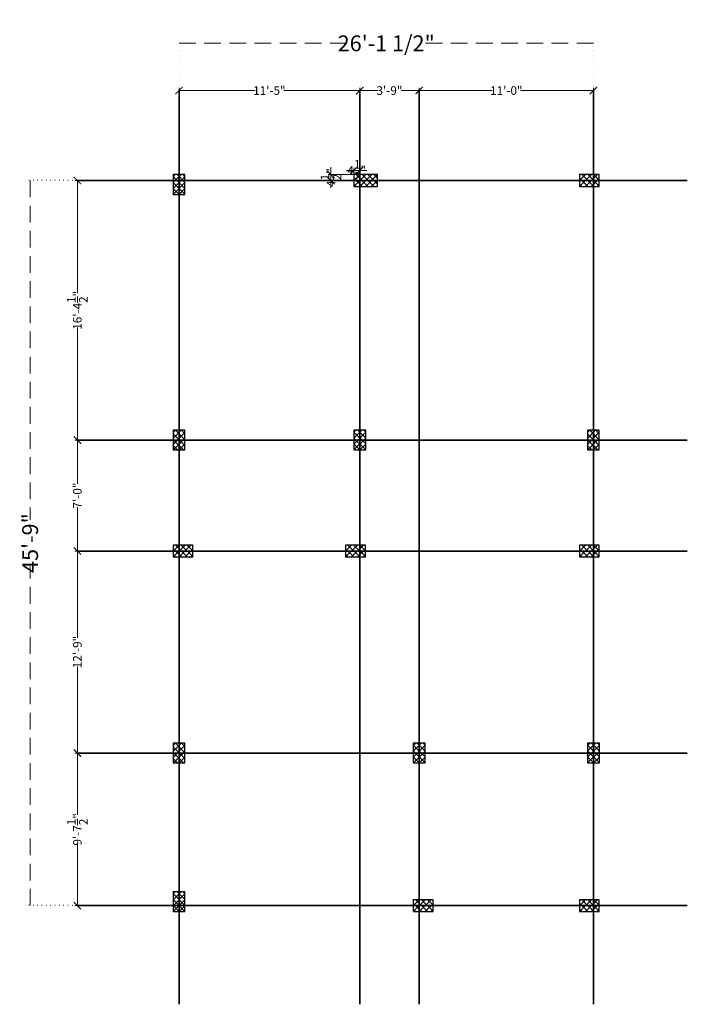
# Model space of a CAD drawing. Units: inches. Extents: x -16911 to -9621, y -48626 to -46270.
# Tile 9 of 20: x -13485 to -12980, y -47015 to -46270. Entities that reach past the tile are written whole.
import ezdxf

# ---------------------------------------------------------------- set-up
doc = ezdxf.new("R2010")
doc.units = ezdxf.units.IN
doc.linetypes.add('DASHED', pattern=[19.05, 12.7, -6.35])
doc.linetypes.add('DOT2', pattern=[3.175, 0, -3.175])
for name, color, linetype, lineweight in [('A-ANNO-DIMS', 2, 'Continuous', 13), ('A-WALL', 7, 'Continuous', 35), ('column', 12, 'Continuous', 30), ('S-COLS', 1, 'Continuous', 30)]:
    doc.layers.add(name, color=color, linetype=linetype, lineweight=lineweight)
doc.styles.add('style3', font='times.ttf')
doc.styles.add('style9', font='swisscl.ttf', dxfattribs={"height": 12})
doc.dimstyles.new('Dim9', dxfattribs={"dimtxt": 10, "dimasz": 0.199219, "dimexe": 1, "dimexo": 0.5, "dimgap": 1, "dimtad": 0, "dimdec": 1, "dimzin": 0, "dimdsep": 46, "dimlunit": 4, "dimtxsty": 'style9', "dimblk": 'ARCHTICK', "dimcen": 0.09, "dimclrd": 256, "dimclrt": 256, "dimadec": 0, "dimazin": 0, "dimtfac": 1, "dimtdec": 1, "dimtix": 1, "dimtofl": 0, "dimtmove": 1, "dimatfit": 3, "dimfxl": 9, "dimtolj": 1, "dimtzin": 0, "dimlwd": -1, "dimarcsym": 0})
doc.dimstyles.new('S.S.S', dxfattribs={"dimtxt": 6.5, "dimasz": 5.5, "dimexe": 2, "dimexo": 0, "dimgap": 0.09, "dimtad": 0, "dimdec": 1, "dimzin": 3, "dimdsep": 46, "dimlunit": 4, "dimtxsty": 'style3', "dimblk": 'ARCHTICK', "dimcen": 2.5, "dimclrd": 252, "dimclre": 256, "dimclrt": 7, "dimadec": 0, "dimazin": 0, "dimtfac": 1, "dimtdec": 1, "dimtix": 1, "dimtofl": 0, "dimtmove": 0, "dimatfit": 3, "dimfxl": 2, "dimtolj": 1, "dimtzin": 0, "dimlwd": 13, "dimlwe": 15, "dimarcsym": 0})

# ---------------------------------------------------------------- blocks, each defined once
blk = doc.blocks.new('COLUMNS')
at = {"layer": 'column'}
h = blk.add_hatch(dxfattribs=at)
h.set_pattern_fill('ANSI37', color=256, angle=-720)
h.set_pattern_definition([(45, (21703.4588, -104481.6704), (-2.24506403, 2.24506403), []), (135, (21703.4588, -104481.6704), (-2.24506403, -2.24506403), [])])
h.paths.add_polyline_path([(-12061.47, -46401.86), (-12052.47, -46401.86), (-12052.47, -46386.86), (-12061.47, -46386.86)])
h = blk.add_hatch(dxfattribs=at)
h.set_pattern_fill('ANSI37', color=256, angle=-810)
h.set_pattern_definition([(315, (-70004.5392, -80151.7886), (2.24506403, 2.24506403), []), (45, (-70004.5392, -80151.7886), (-2.24506403, 2.24506403), [])])
h.paths.add_polyline_path([(-11924.72, -46386.86), (-11924.72, -46395.86), (-11906.72, -46395.86), (-11906.72, -46386.86)])
h = blk.add_hatch(dxfattribs=at)
h.set_pattern_fill('ANSI37', color=256, angle=-810)
h.set_pattern_definition([(315, (-69833.7395, -80151.7886), (2.24506403, 2.24506403), []), (45, (-69833.7395, -80151.7886), (-2.24506403, 2.24506403), [])])
h.paths.add_polyline_path([(-11753.92, -46386.86), (-11753.92, -46395.86), (-11738.92, -46395.86), (-11738.92, -46386.86)])
h = blk.add_hatch(dxfattribs=at)
h.set_pattern_fill('ANSI37', color=256, angle=-900)
h.set_pattern_definition([(225, (-45817.4075, 11499.4594), (2.24506403, -2.24506403), []), (315, (-45817.4075, 11499.4594), (2.24506403, 2.24506403), [])])
h.paths.add_polyline_path([(-12052.47, -46580.36), (-12061.47, -46580.36), (-12061.47, -46595.36), (-12052.47, -46595.36)])
h = blk.add_hatch(dxfattribs=at)
h.set_pattern_fill('ANSI37', color=256, angle=-720)
h.set_pattern_definition([(45, (21840.2088, -104675.1704), (-2.24506403, 2.24506403), []), (135, (21840.2088, -104675.1704), (-2.24506403, -2.24506403), [])])
h.paths.add_polyline_path([(-11924.72, -46595.36), (-11915.72, -46595.36), (-11915.72, -46580.36), (-11924.72, -46580.36)])
h = blk.add_hatch(dxfattribs=at)
h.set_pattern_fill('ANSI37', color=256, angle=-900)
h.set_pattern_definition([(225, (-45503.8578, 11499.4594), (2.24506403, -2.24506403), []), (315, (-45503.8578, 11499.4594), (2.24506403, 2.24506403), [])])
h.paths.add_polyline_path([(-11738.92, -46580.36), (-11747.92, -46580.36), (-11747.92, -46595.36), (-11738.92, -46595.36)])
h = blk.add_hatch(dxfattribs=at)
h.set_pattern_fill('ANSI37', color=256, angle=-810)
h.set_pattern_definition([(315, (-70141.2892, -80432.2886), (2.24506403, 2.24506403), []), (45, (-70141.2892, -80432.2886), (-2.24506403, 2.24506403), [])])
h.paths.add_polyline_path([(-12061.47, -46667.36), (-12061.47, -46676.36), (-12046.47, -46676.36), (-12046.47, -46667.36)])
h = blk.add_hatch(dxfattribs=at)
h.set_pattern_fill('ANSI37', color=256, angle=-810)
h.set_pattern_definition([(315, (-70010.7892, -80432.2886), (2.24506403, 2.24506403), []), (45, (-70010.7892, -80432.2886), (-2.24506403, 2.24506403), [])])
h.paths.add_polyline_path([(-11930.97, -46667.36), (-11930.97, -46676.36), (-11915.97, -46676.36), (-11915.97, -46667.36)])
h = blk.add_hatch(dxfattribs=at)
h.set_pattern_fill('ANSI37', color=256, angle=-810)
h.set_pattern_definition([(315, (-69833.7395, -80432.2886), (2.24506403, 2.24506403), []), (45, (-69833.7395, -80432.2886), (-2.24506403, 2.24506403), [])])
h.paths.add_polyline_path([(-11753.92, -46667.36), (-11753.92, -46676.36), (-11738.92, -46676.36), (-11738.92, -46667.36)])
h = blk.add_hatch(dxfattribs=at)
h.set_pattern_fill('ANSI37', color=256, angle=-540)
h.set_pattern_definition([(225, (-45817.4075, 11262.5055), (2.24506403, -2.24506403), []), (315, (-45817.4075, 11262.5055), (2.24506403, 2.24506403), [])])
h.paths.add_polyline_path([(-12052.47, -46817.31), (-12061.47, -46817.31), (-12061.47, -46832.31), (-12052.47, -46832.31)])
h = blk.add_hatch(dxfattribs=at)
h.set_pattern_fill('ANSI37', color=256, angle=-720)
h.set_pattern_definition([(45, (21885.2088, -104912.1242), (-2.24506403, 2.24506403), []), (135, (21885.2088, -104912.1242), (-2.24506403, -2.24506403), [])])
h.paths.add_polyline_path([(-11879.72, -46832.31), (-11870.72, -46832.31), (-11870.72, -46817.31), (-11879.72, -46817.31)])
h = blk.add_hatch(dxfattribs=at)
h.set_pattern_fill('ANSI37', color=256, angle=-720)
h.set_pattern_definition([(45, (22017.1023, -104912.1242), (-2.24506403, 2.24506403), []), (135, (22017.1023, -104912.1242), (-2.24506403, -2.24506403), [])])
h.paths.add_polyline_path([(-11747.83, -46832.31), (-11738.83, -46832.31), (-11738.83, -46817.31), (-11747.83, -46817.31)])
h = blk.add_hatch(dxfattribs=at)
h.set_pattern_fill('ANSI37', color=256, angle=-720)
h.set_pattern_definition([(45, (21703.4588, -105024.6242), (-2.24506403, 2.24506403), []), (135, (21703.4588, -105024.6242), (-2.24506403, -2.24506403), [])])
h.paths.add_polyline_path([(-12061.47, -46944.81), (-12052.47, -46944.81), (-12052.47, -46929.81), (-12061.47, -46929.81)])
h = blk.add_hatch(dxfattribs=at)
h.set_pattern_fill('ANSI37', color=256, angle=-810)
h.set_pattern_definition([(315, (-69959.5392, -80700.7425), (2.24506403, 2.24506403), []), (45, (-69959.5392, -80700.7425), (-2.24506403, 2.24506403), [])])
h.paths.add_polyline_path([(-11879.72, -46935.81), (-11879.72, -46944.81), (-11864.72, -46944.81), (-11864.72, -46935.81)])
h = blk.add_hatch(dxfattribs=at)
h.set_pattern_fill('ANSI37', color=256, angle=-810)
h.set_pattern_definition([(315, (-69833.7395, -80700.7425), (2.24506403, 2.24506403), []), (45, (-69833.7395, -80700.7425), (-2.24506403, 2.24506403), [])])
h.paths.add_polyline_path([(-11753.92, -46935.81), (-11753.92, -46944.81), (-11738.92, -46944.81), (-11738.92, -46935.81)])
at = {"layer": 'column', "ltscale": 0.05}
for points in [[(-12052.47, -46386.86), (-12061.47, -46386.86), (-12061.47, -46401.86), (-12052.47, -46401.86)], [(-11906.72, -46395.86), (-11906.72, -46386.86), (-11924.72, -46386.86), (-11924.72, -46395.86)], [(-11738.92, -46395.86), (-11738.92, -46386.86), (-11753.92, -46386.86), (-11753.92, -46395.86)], [(-12061.47, -46595.36), (-12052.47, -46595.36), (-12052.47, -46580.36), (-12061.47, -46580.36)], [(-11915.72, -46580.36), (-11924.72, -46580.36), (-11924.72, -46595.36), (-11915.72, -46595.36)], [(-11747.92, -46595.36), (-11738.92, -46595.36), (-11738.92, -46580.36), (-11747.92, -46580.36)], [(-12046.47, -46676.36), (-12046.47, -46667.36), (-12061.47, -46667.36), (-12061.47, -46676.36)], [(-11915.97, -46676.36), (-11915.97, -46667.36), (-11930.97, -46667.36), (-11930.97, -46676.36)], [(-11738.92, -46676.36), (-11738.92, -46667.36), (-11753.92, -46667.36), (-11753.92, -46676.36)], [(-12061.47, -46832.31), (-12052.47, -46832.31), (-12052.47, -46817.31), (-12061.47, -46817.31)], [(-11870.72, -46817.31), (-11879.72, -46817.31), (-11879.72, -46832.31), (-11870.72, -46832.31)], [(-11738.83, -46817.31), (-11747.83, -46817.31), (-11747.83, -46832.31), (-11738.83, -46832.31)], [(-12052.47, -46929.81), (-12061.47, -46929.81), (-12061.47, -46944.81), (-12052.47, -46944.81)], [(-11864.72, -46944.81), (-11864.72, -46935.81), (-11879.72, -46935.81), (-11879.72, -46944.81)], [(-11738.92, -46944.81), (-11738.92, -46935.81), (-11753.92, -46935.81), (-11753.92, -46944.81)]]:
    blk.add_lwpolyline(points, close=True, dxfattribs=at)
blk = doc.blocks.new('_ArchTick')
at = {"color": 0, "linetype": 'ByBlock', "const_width": 0.15}
blk.add_lwpolyline([(-0.5, -0.5), (0.5, 0.5)], dxfattribs=at)
blk = doc.blocks.new('*D33')
at = {"layer": 'A-ANNO-DIMS', "color": 0, "lineweight": 15, "transparency": 16777216}
for p, q in [((-13364.53, -46323.24), (-13364.53, -46321.24)), ((-13227.78, -46323.24), (-13227.78, -46321.24))]:
    blk.add_line(p, q, dxfattribs=at)
at = {"layer": 'A-ANNO-DIMS', "color": 0, "lineweight": 13, "transparency": 16777216}
for p, q in [((-13364.53, -46323.24), (-13306.98, -46323.24)), ((-13227.78, -46323.24), (-13285.32, -46323.24))]:
    blk.add_line(p, q, dxfattribs=at)
at = {"layer": 'Defpoints', "color": 0, "transparency": 16777216}
for p in [(-13364.53, -46323.24), (-13227.78, -46323.24), (-13227.78, -46323.24)]:
    blk.add_point(p, dxfattribs=at)
at = {"layer": 'A-ANNO-DIMS', "color": 0, "lineweight": 13, "transparency": 16777216, "xscale": 5.5, "yscale": 5.5, "zscale": 5.5, "rotation": 180}
blk.add_blockref('_ArchTick', (-13364.53, -46323.24), dxfattribs=at)
at = {"layer": 'A-ANNO-DIMS', "color": 0, "lineweight": 13, "transparency": 16777216, "xscale": 5.5, "yscale": 5.5, "zscale": 5.5}
blk.add_blockref('_ArchTick', (-13227.78, -46323.24), dxfattribs=at)
at = {"layer": 'A-ANNO-DIMS', "color": 0, "transparency": 16777216, "insert": (-13296.15, -46323.24), "char_height": 6.5, "attachment_point": 5, "style": 'style3'}
blk.add_mtext('\\A1;11\'-5"', dxfattribs=at)
blk = doc.blocks.new('*D34')
at = {"layer": 'A-ANNO-DIMS', "color": 0, "lineweight": 15, "transparency": 16777216}
for p, q in [((-13227.78, -46323.24), (-13227.78, -46321.24)), ((-13182.78, -46323.24), (-13182.78, -46321.24))]:
    blk.add_line(p, q, dxfattribs=at)
at = {"layer": 'A-ANNO-DIMS', "color": 0, "lineweight": 13, "transparency": 16777216}
for p, q in [((-13227.78, -46323.24), (-13214.07, -46323.24)), ((-13182.78, -46323.24), (-13196.48, -46323.24))]:
    blk.add_line(p, q, dxfattribs=at)
at = {"layer": 'Defpoints', "color": 0, "transparency": 16777216}
for p in [(-13227.78, -46323.24), (-13182.78, -46323.24), (-13182.78, -46323.24)]:
    blk.add_point(p, dxfattribs=at)
at = {"layer": 'A-ANNO-DIMS', "color": 0, "lineweight": 13, "transparency": 16777216, "xscale": 5.5, "yscale": 5.5, "zscale": 5.5, "rotation": 180}
blk.add_blockref('_ArchTick', (-13227.78, -46323.24), dxfattribs=at)
at = {"layer": 'A-ANNO-DIMS', "color": 0, "lineweight": 13, "transparency": 16777216, "xscale": 5.5, "yscale": 5.5, "zscale": 5.5}
blk.add_blockref('_ArchTick', (-13182.78, -46323.24), dxfattribs=at)
at = {"layer": 'A-ANNO-DIMS', "color": 0, "transparency": 16777216, "insert": (-13205.28, -46323.24), "char_height": 6.5, "attachment_point": 5, "style": 'style3'}
blk.add_mtext('\\A1;3\'-9"', dxfattribs=at)
blk = doc.blocks.new('*D35')
at = {"layer": 'A-ANNO-DIMS', "color": 0, "lineweight": 15, "transparency": 16777216}
for p, q in [((-13182.78, -46323.24), (-13182.78, -46321.24)), ((-13050.88, -46323.24), (-13050.88, -46321.24))]:
    blk.add_line(p, q, dxfattribs=at)
at = {"layer": 'A-ANNO-DIMS', "color": 0, "lineweight": 13, "transparency": 16777216}
for p, q in [((-13182.78, -46323.24), (-13127.66, -46323.24)), ((-13050.88, -46323.24), (-13106, -46323.24))]:
    blk.add_line(p, q, dxfattribs=at)
at = {"layer": 'Defpoints', "color": 0, "transparency": 16777216}
for p in [(-13182.78, -46323.24), (-13050.88, -46323.24), (-13050.88, -46323.24)]:
    blk.add_point(p, dxfattribs=at)
at = {"layer": 'A-ANNO-DIMS', "color": 0, "lineweight": 13, "transparency": 16777216, "xscale": 5.5, "yscale": 5.5, "zscale": 5.5, "rotation": 180}
blk.add_blockref('_ArchTick', (-13182.78, -46323.24), dxfattribs=at)
at = {"layer": 'A-ANNO-DIMS', "color": 0, "lineweight": 13, "transparency": 16777216, "xscale": 5.5, "yscale": 5.5, "zscale": 5.5}
blk.add_blockref('_ArchTick', (-13050.88, -46323.24), dxfattribs=at)
at = {"layer": 'A-ANNO-DIMS', "color": 0, "transparency": 16777216, "insert": (-13116.83, -46323.24), "char_height": 6.5, "attachment_point": 5, "style": 'style3'}
blk.add_mtext('\\A1;11\'-0"', dxfattribs=at)
blk = doc.blocks.new('*D36')
at = {"layer": 'A-ANNO-DIMS', "color": 0, "lineweight": 15, "transparency": 16777216}
for p, q in [((-13441.46, -46824.81), (-13443.46, -46824.81)), ((-13441.46, -46940.31), (-13443.46, -46940.31))]:
    blk.add_line(p, q, dxfattribs=at)
at = {"layer": 'A-ANNO-DIMS', "color": 0, "lineweight": 13, "transparency": 16777216}
for p, q in [((-13441.46, -46824.81), (-13441.46, -46871.49)), ((-13441.46, -46940.31), (-13441.46, -46893.63))]:
    blk.add_line(p, q, dxfattribs=at)
at = {"layer": 'Defpoints', "color": 0, "transparency": 16777216}
for p in [(-13441.46, -46824.81), (-13441.46, -46824.81), (-13441.46, -46940.31)]:
    blk.add_point(p, dxfattribs=at)
at = {"layer": 'A-ANNO-DIMS', "color": 0, "lineweight": 13, "transparency": 16777216, "xscale": 5.5, "yscale": 5.5, "zscale": 5.5}
for p, rotation in [((-13441.46, -46824.81), 90), ((-13441.46, -46940.31), 270)]:
    blk.add_blockref('_ArchTick', p, dxfattribs=dict(at, rotation=rotation))
at = {"layer": 'A-ANNO-DIMS', "color": 0, "transparency": 16777216, "insert": (-13441.46, -46882.56), "char_height": 6.5, "attachment_point": 5, "rotation": 90, "style": 'style3'}
blk.add_mtext('\\A1;9\'-7{\\H1x;\\S1/2;}"', dxfattribs=at)
blk = doc.blocks.new('*D37')
at = {"layer": 'A-ANNO-DIMS', "color": 0, "lineweight": 15, "transparency": 16777216}
for p, q in [((-13441.46, -46671.86), (-13443.46, -46671.86)), ((-13441.46, -46824.81), (-13443.46, -46824.81))]:
    blk.add_line(p, q, dxfattribs=at)
at = {"layer": 'A-ANNO-DIMS', "color": 0, "lineweight": 13, "transparency": 16777216}
for p, q in [((-13441.46, -46671.86), (-13441.46, -46737.5)), ((-13441.46, -46824.81), (-13441.46, -46759.16))]:
    blk.add_line(p, q, dxfattribs=at)
at = {"layer": 'Defpoints', "color": 0, "transparency": 16777216}
for p in [(-13441.46, -46671.86), (-13441.46, -46671.86), (-13441.46, -46824.81)]:
    blk.add_point(p, dxfattribs=at)
at = {"layer": 'A-ANNO-DIMS', "color": 0, "lineweight": 13, "transparency": 16777216, "xscale": 5.5, "yscale": 5.5, "zscale": 5.5}
for p, rotation in [((-13441.46, -46671.86), 90), ((-13441.46, -46824.81), 270)]:
    blk.add_blockref('_ArchTick', p, dxfattribs=dict(at, rotation=rotation))
at = {"layer": 'A-ANNO-DIMS', "color": 0, "transparency": 16777216, "insert": (-13441.46, -46748.33), "char_height": 6.5, "attachment_point": 5, "rotation": 90, "style": 'style3'}
blk.add_mtext('\\A1;12\'-9"', dxfattribs=at)
blk = doc.blocks.new('*D38')
at = {"layer": 'A-ANNO-DIMS', "color": 0, "lineweight": 15, "transparency": 16777216}
for p, q in [((-13441.46, -46587.86), (-13443.46, -46587.86)), ((-13441.46, -46671.86), (-13443.46, -46671.86))]:
    blk.add_line(p, q, dxfattribs=at)
at = {"layer": 'A-ANNO-DIMS', "color": 0, "lineweight": 13, "transparency": 16777216}
for p, q in [((-13441.46, -46587.86), (-13441.46, -46621.04)), ((-13441.46, -46671.86), (-13441.46, -46638.67))]:
    blk.add_line(p, q, dxfattribs=at)
at = {"layer": 'Defpoints', "color": 0, "transparency": 16777216}
for p in [(-13441.46, -46587.86), (-13441.46, -46587.86), (-13441.46, -46671.86)]:
    blk.add_point(p, dxfattribs=at)
at = {"layer": 'A-ANNO-DIMS', "color": 0, "lineweight": 13, "transparency": 16777216, "xscale": 5.5, "yscale": 5.5, "zscale": 5.5}
for p, rotation in [((-13441.46, -46587.86), 90), ((-13441.46, -46671.86), 270)]:
    blk.add_blockref('_ArchTick', p, dxfattribs=dict(at, rotation=rotation))
at = {"layer": 'A-ANNO-DIMS', "color": 0, "transparency": 16777216, "insert": (-13441.46, -46629.86), "char_height": 6.5, "attachment_point": 5, "rotation": 90, "style": 'style3'}
blk.add_mtext('\\A1;7\'-0"', dxfattribs=at)
blk = doc.blocks.new('*D39')
at = {"layer": 'A-ANNO-DIMS', "color": 0, "lineweight": 15, "transparency": 16777216}
for p, q in [((-13441.46, -46391.36), (-13443.46, -46391.36)), ((-13441.46, -46587.86), (-13443.46, -46587.86))]:
    blk.add_line(p, q, dxfattribs=at)
at = {"layer": 'A-ANNO-DIMS', "color": 0, "lineweight": 13, "transparency": 16777216}
for p, q in [((-13441.46, -46391.36), (-13441.46, -46476.51)), ((-13441.46, -46587.86), (-13441.46, -46502.7))]:
    blk.add_line(p, q, dxfattribs=at)
at = {"layer": 'Defpoints', "color": 0, "transparency": 16777216}
for p in [(-13441.46, -46391.36), (-13441.46, -46391.36), (-13441.46, -46587.86)]:
    blk.add_point(p, dxfattribs=at)
at = {"layer": 'A-ANNO-DIMS', "color": 0, "lineweight": 13, "transparency": 16777216, "xscale": 5.5, "yscale": 5.5, "zscale": 5.5}
for p, rotation in [((-13441.46, -46391.36), 90), ((-13441.46, -46587.86), 270)]:
    blk.add_blockref('_ArchTick', p, dxfattribs=dict(at, rotation=rotation))
at = {"layer": 'A-ANNO-DIMS', "color": 0, "transparency": 16777216, "insert": (-13441.46, -46489.61), "char_height": 6.5, "attachment_point": 5, "rotation": 90, "style": 'style3'}
blk.add_mtext('\\A1;16\'-4{\\H1x;\\S1/2;}"', dxfattribs=at)
blk = doc.blocks.new('*D50')
at = {"layer": 'A-ANNO-DIMS', "color": 0, "lineweight": 13, "transparency": 16777216}
for p, q in [((-13232.28, -46383.67), (-13237.78, -46383.67)), ((-13227.78, -46383.67), (-13222.28, -46383.67))]:
    blk.add_line(p, q, dxfattribs=at)
at = {"layer": 'A-ANNO-DIMS', "color": 0, "lineweight": 15, "transparency": 16777216}
for p, q in [((-13232.28, -46386.86), (-13232.28, -46381.67)), ((-13227.78, -46386.86), (-13227.78, -46381.67))]:
    blk.add_line(p, q, dxfattribs=at)
at = {"layer": 'Defpoints', "color": 0, "transparency": 16777216}
for p in [(-13232.28, -46383.67), (-13232.28, -46386.86), (-13227.78, -46386.86)]:
    blk.add_point(p, dxfattribs=at)
at = {"layer": 'A-ANNO-DIMS', "color": 0, "lineweight": 13, "transparency": 16777216, "xscale": 5.5, "yscale": 5.5, "zscale": 5.5}
blk.add_blockref('_ArchTick', (-13232.28, -46383.67), dxfattribs=at)
at = {"layer": 'A-ANNO-DIMS', "color": 0, "lineweight": 13, "transparency": 16777216, "xscale": 5.5, "yscale": 5.5, "zscale": 5.5, "rotation": 180}
blk.add_blockref('_ArchTick', (-13227.78, -46383.67), dxfattribs=at)
at = {"layer": 'A-ANNO-DIMS', "color": 0, "transparency": 16777216, "insert": (-13230.03, -46383.67), "char_height": 6.5, "attachment_point": 5, "style": 'style3'}
blk.add_mtext('\\A1;4{\\H1x;\\S1/2;}"', dxfattribs=at)
blk = doc.blocks.new('*D51')
at = {"layer": 'A-ANNO-DIMS', "color": 0, "lineweight": 15, "transparency": 16777216}
for p, q in [((-13232.28, -46386.86), (-13251.58, -46386.86)), ((-13232.28, -46391.36), (-13251.58, -46391.36))]:
    blk.add_line(p, q, dxfattribs=at)
at = {"layer": 'A-ANNO-DIMS', "color": 0, "lineweight": 13, "transparency": 16777216}
for p, q in [((-13249.58, -46386.86), (-13249.58, -46381.36)), ((-13249.58, -46391.36), (-13249.58, -46396.86))]:
    blk.add_line(p, q, dxfattribs=at)
at = {"layer": 'Defpoints', "color": 0, "transparency": 16777216}
for p in [(-13232.28, -46386.86), (-13249.58, -46391.36), (-13232.28, -46391.36)]:
    blk.add_point(p, dxfattribs=at)
at = {"layer": 'A-ANNO-DIMS', "color": 0, "lineweight": 13, "transparency": 16777216, "xscale": 5.5, "yscale": 5.5, "zscale": 5.5}
for p, rotation in [((-13249.58, -46386.86), 270), ((-13249.58, -46391.36), 90)]:
    blk.add_blockref('_ArchTick', p, dxfattribs=dict(at, rotation=rotation))
at = {"layer": 'A-ANNO-DIMS', "color": 0, "transparency": 16777216, "insert": (-13249.58, -46389.11), "char_height": 6.5, "attachment_point": 5, "rotation": 90, "style": 'style3'}
blk.add_mtext('\\A1;4{\\H1x;\\S1/2;}"', dxfattribs=at)
blk = doc.blocks.new('*D133')
at = {"layer": 'A-ANNO-DIMS', "color": 0, "linetype": 'DOT2', "lineweight": -2, "transparency": 16777216}
for p, q in [((-13364.53, -46322.74), (-13364.53, -46286.49)), ((-13050.88, -46322.74), (-13050.88, -46286.49))]:
    blk.add_line(p, q, dxfattribs=at)
at = {"layer": 'A-ANNO-DIMS', "linetype": 'DASHED', "transparency": 16777216}
for p, q in [((-13364.53, -46287.49), (-13236.95, -46287.49)), ((-13050.88, -46287.49), (-13178.45, -46287.49))]:
    blk.add_line(p, q, dxfattribs=at)
at = {"layer": 'Defpoints', "color": 0, "transparency": 16777216}
for p in [(-13050.88, -46287.49), (-13364.53, -46323.24), (-13050.88, -46323.24)]:
    blk.add_point(p, dxfattribs=at)
at = {"layer": 'A-ANNO-DIMS', "transparency": 16777216, "xscale": 0.19921875, "yscale": 0.19921875, "zscale": 0.19921875, "rotation": 180}
blk.add_blockref('_ArchTick', (-13364.53, -46287.49), dxfattribs=at)
at = {"layer": 'A-ANNO-DIMS', "transparency": 16777216, "xscale": 0.19921875, "yscale": 0.19921875, "zscale": 0.19921875}
blk.add_blockref('_ArchTick', (-13050.88, -46287.49), dxfattribs=at)
at = {"layer": 'A-ANNO-DIMS', "transparency": 16777216, "insert": (-13207.7, -46287.49), "char_height": 12, "attachment_point": 5, "style": 'style9'}
blk.add_mtext('\\A1;26\'-1 1/2"', dxfattribs=at)
blk = doc.blocks.new('*D134')
at = {"layer": 'A-ANNO-DIMS', "color": 0, "linetype": 'DOT2', "lineweight": -2, "transparency": 16777216}
for p, q in [((-13441.96, -46391.36), (-13478.21, -46391.36)), ((-13441.96, -46940.31), (-13478.21, -46940.31))]:
    blk.add_line(p, q, dxfattribs=at)
at = {"layer": 'A-ANNO-DIMS', "linetype": 'DASHED', "transparency": 16777216}
for p, q in [((-13477.21, -46391.36), (-13477.21, -46648.2)), ((-13477.21, -46940.31), (-13477.21, -46683.47))]:
    blk.add_line(p, q, dxfattribs=at)
at = {"layer": 'Defpoints', "color": 0, "transparency": 16777216}
for p in [(-13441.46, -46391.36), (-13477.21, -46940.31), (-13441.46, -46940.31)]:
    blk.add_point(p, dxfattribs=at)
at = {"layer": 'A-ANNO-DIMS', "transparency": 16777216, "xscale": 0.19921875, "yscale": 0.19921875, "zscale": 0.19921875}
for p, rotation in [((-13477.21, -46391.36), 90), ((-13477.21, -46940.31), 270)]:
    blk.add_blockref('_ArchTick', p, dxfattribs=dict(at, rotation=rotation))
at = {"layer": 'A-ANNO-DIMS', "transparency": 16777216, "insert": (-13477.21, -46665.83), "char_height": 12, "attachment_point": 5, "rotation": 90, "style": 'style9'}
blk.add_mtext('\\A1;45\'-9"', dxfattribs=at)

msp = doc.modelspace()

# ---------------------------------------------------------------- linework, layer by layer
at = {"layer": 'A-WALL'}
for p, q in [((-13364.525, -46323.239), (-13364.525, -47015.019)), ((-13227.775, -46323.239), (-13227.775, -47015.019)), ((-13182.775, -46323.239), (-13182.775, -47015.019)), ((-13050.882, -46323.239), (-13050.882, -47015.019)), ((-13441.459, -46391.355), (-12979.873, -46391.355)), ((-13441.459, -46587.855), (-12979.873, -46587.855)), ((-13441.459, -46671.855), (-12979.873, -46671.855)), ((-13441.459, -46824.809), (-12979.873, -46824.809)), ((-13441.459, -46940.309), (-12979.873, -46940.309))]:
    msp.add_line(p, q, dxfattribs=at)

# ---------------------------------------------------------------- block references
at = {"layer": 'S-COLS'}
msp.add_blockref('COLUMNS', (-1307.551, 0), dxfattribs=at)

# ---------------------------------------------------------------- dimensions: what is measured, and where the dimension line sits
at = {"layer": 'A-ANNO-DIMS'}
for base, p1, p2, dimstyle, override, picture, middle in [((-13050.882, -46287.489), (-13364.525, -46323.239), (-13050.882, -46323.239), 'Dim9', {"dimdec": 1, "dimlfac": 1, "dimrnd": 0, "dimzin": 1, "dimdsep": 46, "dimlunit": 4, "dimfrac": 2}, '*D133', (-13207.704, -46287.489)), ((-13227.775423602, -46323.239487031), (-13364.525423602, -46323.239487031), (-13227.775423602, -46323.239487031), 'S.S.S', {"dimclrd": 0, "dimclre": 0, "dimclrt": 0}, '*D33', (-13296.150423602, -46323.239487031)), ((-13182.775, -46323.239), (-13227.775, -46323.239), (-13182.775, -46323.239), 'S.S.S', {"dimclrd": 0, "dimclre": 0, "dimclrt": 0, "dimtmove": 1}, '*D34', (-13205.275, -46323.239)), ((-13050.882, -46323.239), (-13182.775, -46323.239), (-13050.882, -46323.239), 'S.S.S', {"dimclrd": 0, "dimclre": 0, "dimclrt": 0, "dimtmove": 1}, '*D35', (-13116.829, -46323.239)), ((-13232.275, -46383.666), (-13227.775, -46386.855), (-13232.275, -46386.855), 'S.S.S', {"dimclrd": 0, "dimclre": 0, "dimclrt": 0}, '*D50', (-13230.025, -46383.666))]:
    dim = msp.add_linear_dim(base=base, p1=p1, p2=p2, dimstyle=dimstyle, override=override, dxfattribs=at)
    dim.commit()
    dim.dimension.update_dxf_attribs({"geometry": picture, "text_midpoint": middle})
for base, p1, p2, dimstyle, override, picture, middle in [((-13249.582, -46391.355), (-13232.275, -46386.855), (-13232.275, -46391.355), 'S.S.S', {"dimclrd": 0, "dimclre": 0, "dimclrt": 0}, '*D51', (-13249.582, -46389.105)), ((-13477.209, -46940.309), (-13441.459, -46391.355), (-13441.459, -46940.309), 'Dim9', {"dimdec": 1, "dimlfac": 1, "dimrnd": 0, "dimzin": 1, "dimdsep": 46, "dimlunit": 4, "dimfrac": 2}, '*D134', (-13477.209, -46665.832)), ((-13441.459, -46391.355), (-13441.459, -46587.855), (-13441.459, -46391.355), 'S.S.S', {"dimclrd": 0, "dimclre": 0, "dimclrt": 0, "dimtmove": 1}, '*D39', (-13441.459, -46489.605)), ((-13441.459, -46587.855), (-13441.459, -46671.855), (-13441.459, -46587.855), 'S.S.S', {"dimclrd": 0, "dimclre": 0, "dimclrt": 0, "dimtmove": 1}, '*D38', (-13441.459, -46629.855)), ((-13441.459, -46671.855), (-13441.459, -46824.809), (-13441.459, -46671.855), 'S.S.S', {"dimclrd": 0, "dimclre": 0, "dimclrt": 0, "dimtmove": 1}, '*D37', (-13441.459, -46748.332)), ((-13441.459, -46824.809), (-13441.459, -46940.309), (-13441.459, -46824.809), 'S.S.S', {"dimclrd": 0, "dimclre": 0, "dimclrt": 0}, '*D36', (-13441.459, -46882.559))]:
    dim = msp.add_linear_dim(base=base, p1=p1, p2=p2, angle=90, dimstyle=dimstyle, override=override, dxfattribs=at)
    dim.commit()
    dim.dimension.update_dxf_attribs({"geometry": picture, "text_midpoint": middle})

doc.saveas('drawing.dxf')
